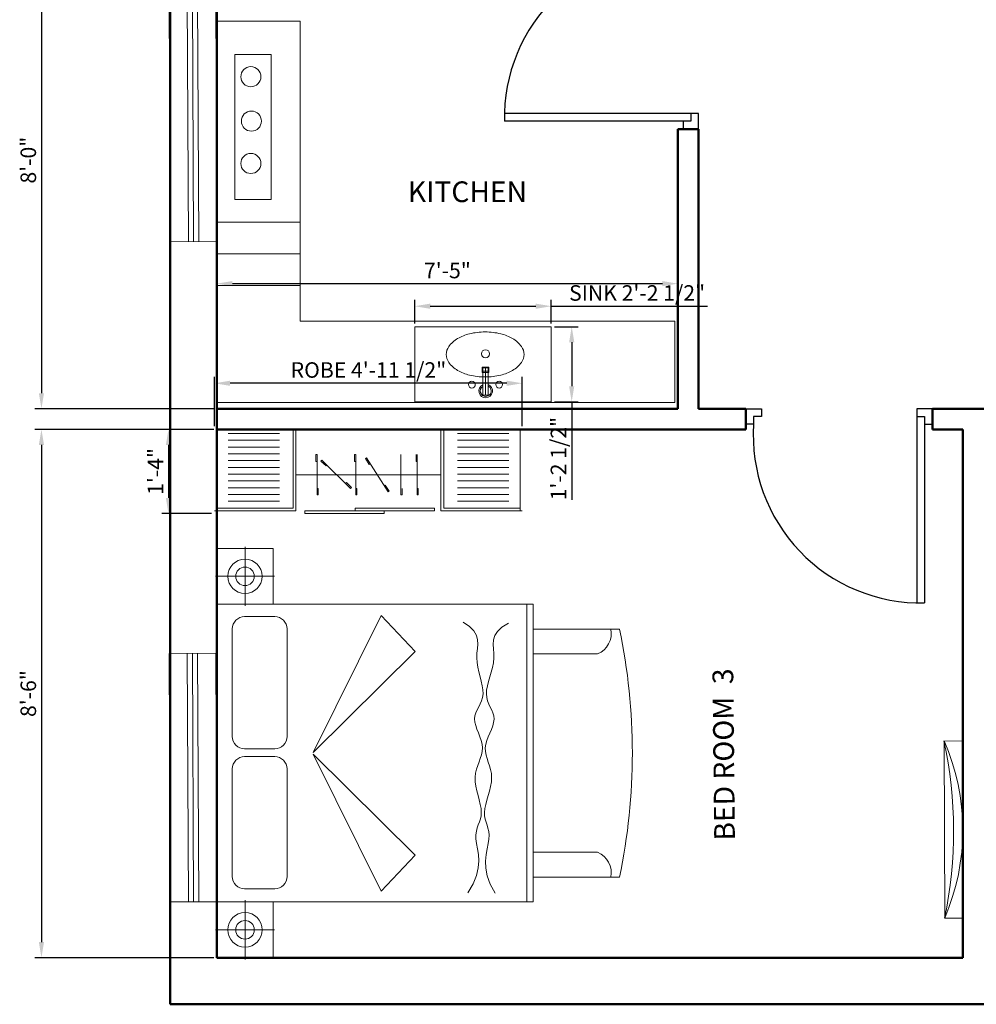
# Model space of a CAD drawing. Units: inches. Extents: x 108 to 1546, y -229 to 513.
# Tile 8 of 11: x 1167 to 1352, y -4 to 187. Entities that reach past the tile are written whole.
import ezdxf

# ---------------------------------------------------------------- set-up
doc = ezdxf.new("R2010")
doc.units = ezdxf.units.IN
for name, color, linetype, lineweight in [('A-ANNO-DIMS', 2, 'Continuous', 18), ('A-AREA-IDEN', 4, 'Continuous', 18), ('A-EQPM', 8, 'Continuous', 18), ('A-FLOR-CBNT', 8, 'Continuous', 18), ('A-FLOR-FIXT', 9, 'Continuous', 18), ('A-FURN', 8, 'Continuous', 13), ('door', 1, 'Continuous', 25), ('tv', 2, 'Continuous', 13), ('wall', 7, 'Continuous', 50), ('WINDOW', 212, 'Continuous', 18)]:
    doc.layers.add(name, color=color, linetype=linetype, lineweight=lineweight)
doc.styles.get("Standard").update_dxf_attribs({"font": 'arial.ttf'})
doc.dimstyles.new('ISO-25', dxfattribs={"dimtxt": 3, "dimasz": 3, "dimexe": 1.25, "dimexo": 0.625, "dimtad": 1, "dimdec": 1, "dimlunit": 3, "dimtxsty": 'Standard', "dimcen": 2.5, "dimadec": 0, "dimazin": 0, "dimtfac": 1, "dimtdec": 1, "dimtmove": 0, "dimatfit": 3, "dimfxl": 1, "dimarcsym": 0})

# ---------------------------------------------------------------- blocks, each defined once
blk = doc.blocks.new('A$C4F543DC7')
for p, q in [((0.0134, 3.35, -0.1688), (3.3134, 3.35, -0.1688)), ((0.4634, 3.35, -0.1688), (0.0134, 3.35, -0.1688)), ((0.0134, 2.896, -0.1688), (0.0134, 3.35, -0.1688)), ((0.0134, 3.35, -0.1688), (0.0134, 2.896, -0.1688)), ((0.2381, 3.1233, -0.4388), (0.2381, 3.3614, -0.4388)), ((0.4634, 3.35, -0.1688), (0.4634, 0.8, -0.1688)), ((2.8634, 3.35, -0.1688), (0.4634, 3.35, -0.1688)), ((0.4634, 2.896, -0.1688), (0.4634, 3.35, -0.1688)), ((2.8634, 0.8, -0.1688), (2.8634, 3.35, -0.1688)), ((2.8634, 3.35, -0.1688), (3.3134, 3.35, -0.1688)), ((2.8634, 2.896, -0.1688), (2.8634, 3.35, -0.1688)), ((3.0888, 3.1233, -0.4388), (3.0888, 3.3614, -0.4388)), ((3.3134, 3.35, -0.1688), (3.3134, 2.896, -0.1688)), ((3.3134, 3.35, -0.1688), (3.3134, 2.896, -0.1688)), ((1.5354, 3.226, -0.1688), (0.6684, 3.226, -0.1688)), ((2.6644, 3.226, -0.1688), (1.7974, 3.226, -0.1688)), ((0.2381, 3.1233, -0.4388), (0, 3.1233, -0.4388)), ((0.2381, 3.1233, -0.4388), (0.4762, 3.1233, -0.4388)), ((0.2381, 3.1233, -0.4388), (0.2381, 2.8852, -0.4388)), ((0.5684, 3.126, -0.1688), (0.5684, 2.884, -0.1688)), ((1.6354, 2.884, -0.1688), (1.6354, 3.126, -0.1688)), ((1.6974, 3.126, -0.1688), (1.6974, 2.884, -0.1688)), ((2.7644, 2.884, -0.1688), (2.7644, 3.126, -0.1688)), ((3.0888, 3.1233, -0.4388), (2.8507, 3.1233, -0.4388)), ((3.0888, 3.1233, -0.4388), (3.0888, 2.8852, -0.4388)), ((3.0888, 3.1233, -0.4388), (3.3269, 3.1233, -0.4388)), ((0.4634, 2.896, -0.1688), (0.0134, 2.896, -0.1688)), ((0.0134, 2.896, -0.1688), (0.4634, 2.896, -0.1688)), ((0.4634, 0.8, -0.1688), (0.4634, 2.896, -0.1688)), ((2.8634, 2.896, -0.1688), (2.8634, 0.8, -0.1688)), ((3.3134, 2.896, -0.1688), (2.8634, 2.896, -0.1688)), ((3.3134, 2.896, -0.1688), (2.8634, 2.896, -0.1688)), ((0.6684, 2.784, -0.1688), (1.5354, 2.784, -0.1688)), ((1.7974, 2.784, -0.1688), (2.6644, 2.784, -0.1688)), ((1.6534, 2.573, -0.1688), (0.5504, 2.025, -0.1688)), ((0.8414, 1.752, -0.1688), (1.6534, 2.573, -0.1688)), ((2.4814, 1.752, -0.1688), (1.6694, 2.573, -0.1688)), ((1.6694, 2.573, -0.1688), (2.7724, 2.025, -0.1688)), ((0.5504, 2.025, -0.1688), (0.8414, 1.752, -0.1688)), ((2.7724, 2.025, -0.1688), (2.4814, 1.752, -0.1688)), ((2.683, 1.312, -0.1688), (2.7182, 1.3641, -0.1688)), ((0.5369, 1.3267, -0.1688), (0.6088, 1.2835, -0.1688)), ((0.6088, 1.2835, -0.1688), (0.6756, 1.2566, -0.1688)), ((1.913, 1.2698, -0.1688), (1.9397, 1.2722, -0.1688)), ((1.9397, 1.2722, -0.1688), (1.9649, 1.2692, -0.1688)), ((2.6129, 1.257, -0.1688), (2.6479, 1.2774, -0.1688)), ((2.6479, 1.2774, -0.1688), (2.683, 1.312, -0.1688)), ((0.6756, 1.2566, -0.1688), (0.7373, 1.2428, -0.1688)), ((0.7373, 1.2428, -0.1688), (0.794, 1.239, -0.1688)), ((0.794, 1.239, -0.1688), (0.8457, 1.242, -0.1688)), ((0.8457, 1.242, -0.1688), (0.8925, 1.2489, -0.1688)), ((0.8925, 1.2489, -0.1688), (0.9345, 1.2564, -0.1688)), ((0.9345, 1.2564, -0.1688), (0.9718, 1.2615, -0.1688)), ((0.9718, 1.2615, -0.1688), (1.0044, 1.2617, -0.1688)), ((1.0044, 1.2617, -0.1688), (1.0334, 1.2578, -0.1688)), ((1.0334, 1.2578, -0.1688), (1.0597, 1.2509, -0.1688)), ((1.0597, 1.2509, -0.1688), (1.0842, 1.2424, -0.1688)), ((1.0842, 1.2424, -0.1688), (1.1081, 1.2336, -0.1688)), ((1.1081, 1.2336, -0.1688), (1.1322, 1.2257, -0.1688)), ((1.1316, 1.1872, -0.1688), (1.1573, 1.192, -0.1688)), ((1.1322, 1.2257, -0.1688), (1.1577, 1.2201, -0.1688)), ((1.1573, 1.192, -0.1688), (1.1851, 1.1932, -0.1688)), ((1.1577, 1.2201, -0.1688), (1.1855, 1.218, -0.1688)), ((1.1851, 1.1932, -0.1688), (1.2158, 1.1898, -0.1688)), ((1.1855, 1.218, -0.1688), (1.2163, 1.2204, -0.1688)), ((1.2163, 1.2204, -0.1688), (1.2498, 1.2264, -0.1688)), ((1.2498, 1.2264, -0.1688), (1.2852, 1.2347, -0.1688)), ((1.2852, 1.2347, -0.1688), (1.3218, 1.2441, -0.1688)), ((1.3218, 1.2441, -0.1688), (1.3591, 1.2533, -0.1688)), ((1.3591, 1.2533, -0.1688), (1.3963, 1.2612, -0.1688)), ((1.3963, 1.2612, -0.1688), (1.4328, 1.2664, -0.1688)), ((1.4328, 1.2664, -0.1688), (1.4679, 1.2677, -0.1688)), ((1.4679, 1.2677, -0.1688), (1.501, 1.2643, -0.1688)), ((1.501, 1.2643, -0.1688), (1.5324, 1.257, -0.1688)), ((1.5324, 1.257, -0.1688), (1.5624, 1.2473, -0.1688)), ((1.5624, 1.2473, -0.1688), (1.5915, 1.2365, -0.1688)), ((1.5915, 1.2365, -0.1688), (1.6199, 1.2259, -0.1688)), ((1.6199, 1.2259, -0.1688), (1.6481, 1.2169, -0.1688)), ((1.6481, 1.2169, -0.1688), (1.6765, 1.2108, -0.1688)), ((1.6765, 1.2108, -0.1688), (1.7053, 1.209, -0.1688)), ((1.7053, 1.209, -0.1688), (1.7349, 1.2124, -0.1688)), ((1.7349, 1.2124, -0.1688), (1.7651, 1.2199, -0.1688)), ((1.7651, 1.2199, -0.1688), (1.7955, 1.2301, -0.1688)), ((1.7955, 1.2301, -0.1688), (1.8258, 1.2417, -0.1688)), ((1.8258, 1.2417, -0.1688), (1.8557, 1.2531, -0.1688)), ((1.8557, 1.2531, -0.1688), (1.8849, 1.263, -0.1688)), ((1.8849, 1.263, -0.1688), (1.913, 1.2698, -0.1688)), ((1.9649, 1.2692, -0.1688), (1.989, 1.2617, -0.1688)), ((1.989, 1.2617, -0.1688), (2.0124, 1.2512, -0.1688)), ((2.0124, 1.2512, -0.1688), (2.0359, 1.2391, -0.1688)), ((2.0359, 1.2391, -0.1688), (2.0599, 1.2269, -0.1688)), ((2.0599, 1.2269, -0.1688), (2.0849, 1.216, -0.1688)), ((2.0849, 1.216, -0.1688), (2.1117, 1.2077, -0.1688)), ((2.1117, 1.2077, -0.1688), (2.1407, 1.2037, -0.1688)), ((2.1407, 1.2037, -0.1688), (2.1723, 1.2047, -0.1688)), ((2.1723, 1.2047, -0.1688), (2.2062, 1.21, -0.1688)), ((2.2062, 1.21, -0.1688), (2.242, 1.2182, -0.1688)), ((2.242, 1.2182, -0.1688), (2.2791, 1.2279, -0.1688)), ((2.2791, 1.2279, -0.1688), (2.3173, 1.2378, -0.1688)), ((2.3173, 1.2378, -0.1688), (2.3558, 1.2465, -0.1688)), ((2.3558, 1.2465, -0.1688), (2.3944, 1.2527, -0.1688)), ((2.3944, 1.2527, -0.1688), (2.4325, 1.255, -0.1688)), ((2.4325, 1.255, -0.1688), (2.4698, 1.2529, -0.1688)), ((2.4698, 1.2529, -0.1688), (2.5064, 1.2488, -0.1688)), ((2.5064, 1.2488, -0.1688), (2.5423, 1.2459, -0.1688)), ((2.5423, 1.2459, -0.1688), (2.5777, 1.2476, -0.1688)), ((2.5777, 1.2476, -0.1688), (2.6129, 1.257, -0.1688)), ((0.5334, 1.105, -0.1688), (0.6067, 1.1458, -0.1688)), ((0.6067, 1.1458, -0.1688), (0.6743, 1.1706, -0.1688)), ((0.6743, 1.1706, -0.1688), (0.7364, 1.1825, -0.1688)), ((0.7364, 1.1825, -0.1688), (0.7931, 1.1846, -0.1688)), ((0.7931, 1.1846, -0.1688), (0.8447, 1.1799, -0.1688)), ((0.8447, 1.1799, -0.1688), (0.8913, 1.1716, -0.1688)), ((0.8913, 1.1716, -0.1688), (0.9331, 1.1628, -0.1688)), ((0.9331, 1.1628, -0.1688), (0.9701, 1.1565, -0.1688)), ((0.9701, 1.1565, -0.1688), (1.0027, 1.1552, -0.1688)), ((1.0027, 1.1552, -0.1688), (1.0318, 1.1582, -0.1688)), ((1.0318, 1.1582, -0.1688), (1.0583, 1.1642, -0.1688)), ((1.0583, 1.1642, -0.1688), (1.0831, 1.172, -0.1688)), ((1.0831, 1.172, -0.1688), (1.1072, 1.18, -0.1688)), ((1.1072, 1.18, -0.1688), (1.1316, 1.1872, -0.1688)), ((1.2158, 1.1898, -0.1688), (1.2491, 1.1828, -0.1688)), ((1.2491, 1.1828, -0.1688), (1.2842, 1.1734, -0.1688)), ((1.2842, 1.1734, -0.1688), (1.3206, 1.1629, -0.1688)), ((1.3206, 1.1629, -0.1688), (1.3575, 1.1524, -0.1688)), ((1.3575, 1.1524, -0.1688), (1.3945, 1.1434, -0.1688)), ((1.3945, 1.1434, -0.1688), (1.4308, 1.1371, -0.1688)), ((1.4308, 1.1371, -0.1688), (1.4658, 1.1347, -0.1688)), ((1.4658, 1.1347, -0.1688), (1.499, 1.137, -0.1688)), ((1.499, 1.137, -0.1688), (1.5306, 1.1433, -0.1688)), ((1.5306, 1.1433, -0.1688), (1.5609, 1.152, -0.1688)), ((1.5609, 1.152, -0.1688), (1.5903, 1.1619, -0.1688)), ((1.5903, 1.1619, -0.1688), (1.6191, 1.1716, -0.1688)), ((1.6191, 1.1716, -0.1688), (1.6475, 1.1797, -0.1688)), ((1.6475, 1.1797, -0.1688), (1.676, 1.1849, -0.1688)), ((1.676, 1.1849, -0.1688), (1.7049, 1.1858, -0.1688)), ((1.7049, 1.1858, -0.1688), (1.7344, 1.1816, -0.1688)), ((1.7344, 1.1816, -0.1688), (1.7643, 1.1731, -0.1688)), ((1.7643, 1.1731, -0.1688), (1.7944, 1.1619, -0.1688)), ((1.7944, 1.1619, -0.1688), (1.8244, 1.1494, -0.1688)), ((1.8244, 1.1494, -0.1688), (1.8539, 1.137, -0.1688)), ((1.8539, 1.137, -0.1688), (1.8827, 1.1263, -0.1688)), ((1.8827, 1.1263, -0.1688), (1.9106, 1.1186, -0.1688)), ((1.9106, 1.1186, -0.1688), (1.9373, 1.1153, -0.1688)), ((1.9373, 1.1153, -0.1688), (1.9625, 1.1176, -0.1688)), ((1.9625, 1.1176, -0.1688), (1.9868, 1.1243, -0.1688)), ((1.9868, 1.1243, -0.1688), (2.0106, 1.134, -0.1688)), ((2.0106, 1.134, -0.1688), (2.0344, 1.1454, -0.1688)), ((2.0344, 1.1454, -0.1688), (2.0588, 1.1568, -0.1688)), ((2.0588, 1.1568, -0.1688), (2.0842, 1.167, -0.1688)), ((2.0842, 1.167, -0.1688), (2.1112, 1.1743, -0.1688)), ((2.1112, 1.1743, -0.1688), (2.1403, 1.1775, -0.1688)), ((2.1403, 1.1775, -0.1688), (2.1718, 1.1755, -0.1688)), ((2.1718, 1.1755, -0.1688), (2.2056, 1.1691, -0.1688)), ((2.2056, 1.1691, -0.1688), (2.2411, 1.1598, -0.1688)), ((2.2411, 1.1598, -0.1688), (2.2779, 1.1489, -0.1688)), ((2.2779, 1.1489, -0.1688), (2.3157, 1.1379, -0.1688)), ((2.3157, 1.1379, -0.1688), (2.354, 1.1279, -0.1688)), ((2.354, 1.1279, -0.1688), (2.3923, 1.1205, -0.1688)), ((2.3923, 1.1205, -0.1688), (2.4304, 1.117, -0.1688)), ((2.4304, 1.117, -0.1688), (2.4677, 1.118, -0.1688)), ((2.4677, 1.118, -0.1688), (2.5043, 1.1209, -0.1688)), ((2.5043, 1.1209, -0.1688), (2.5403, 1.1226, -0.1688)), ((2.5403, 1.1226, -0.1688), (2.5757, 1.1199, -0.1688)), ((2.5757, 1.1199, -0.1688), (2.6106, 1.1094, -0.1688)), ((2.6106, 1.1094, -0.1688), (2.645, 1.0879, -0.1688)), ((2.645, 1.0879, -0.1688), (2.6789, 1.0522, -0.1688)), ((2.6789, 1.0522, -0.1688), (2.7124, 0.999, -0.1688)), ((0.4634, 0.85, -0.1688), (2.8634, 0.85, -0.1688)), ((0.4634, 0.8, -0.1688), (2.8634, 0.8, -0.1688)), ((0.6634, 0.8, -0.1688), (0.4634, 0.8, -0.1688)), ((0.6634, 0.8, -0.1688), (2.6634, 0.8, -0.1688)), ((0.6634, 0.104, -0.1688), (0.6634, 0.8, -0.1688)), ((0.6634, 0.104, -0.1688), (0.6634, 0.8, -0.1688)), ((0.8634, 0.281, -0.1688), (0.8634, 0.8, -0.1688)), ((2.4634, 0.8, -0.1688), (2.4634, 0.281, -0.1688)), ((2.8634, 0.8, -0.1688), (2.6634, 0.8, -0.1688)), ((2.6634, 0.8, -0.1688), (2.6634, 0.104, -0.1688)), ((2.6634, 0.8, -0.1688), (2.6634, 0.104, -0.1688))]:
    blk.add_line(p, q)
for centre, radius in [((0.2381, 3.1233, -0.4388), 0.139), ((3.0888, 3.1233, -0.4388), 0.139), ((0.2381, 3.1233, -0.4388), 0.075), ((3.0888, 3.1233, -0.4388), 0.075)]:
    blk.add_circle(centre, radius)
for centre, radius, start, end in [((0.6684, 3.126, -0.1688), 0.1, 90, 180), ((1.5354, 3.126, -0.1688), 0.1, 0, 90), ((1.7974, 3.126, -0.1688), 0.1, 90, 180), ((2.6644, 3.126, -0.1688), 0.1, 0, 90), ((0.6684, 2.884, -0.1688), 0.1, 180, 270), ((1.5354, 2.884, -0.1688), 0.1, 270, 0), ((1.7974, 2.884, -0.1688), 0.1, 180, 270), ((2.6644, 2.884, -0.1688), 0.1, 270, 0), ((0.6994, 0.3472, -0.1688), 0.1769, 258.2616, 338.03196), ((2.6275, 0.3472, -0.1688), 0.1769, 201.96804, 281.7384), ((1.6634, 4.8597, -0.1688), 4.8597, 258.12517, 281.87483), ((1.6634, 4.8597, -0.1688), 4.8597, 258.12517, 281.87483)]:
    blk.add_arc(centre, radius, start, end)
blk = doc.blocks.new('A$C34930FF8')
at = {"ltscale": 0.05}
for p, q in [((0, 2252.4), (0, 16.8)), ((600, 2252.4), (0, 2252.4)), ((185.4, 1513), (185.4, 1521.5)), ((227.1, 1479.2), (233.2, 1485.2)), ((237.7, 1513), (237.7, 1521.5)), ((436.7, 1513), (436.7, 1504.4)), ((482.5, 1513), (482.5, 1504.4)), ((263.6, 1441.7), (269.7, 1447.7)), ((185.4, 1229.1), (185.4, 1237.7)), ((237.7, 1229.1), (237.7, 1237.7)), ((398.2, 1303.6), (392.1, 1297.6)), ((434.8, 1266.1), (428.7, 1260.1)), ((436.7, 1228.2), (436.7, 1219.7)), ((482.5, 1228.2), (482.5, 1219.7)), ((209.5, 1150.1), (214.1, 1157.3)), ((253.5, 1121.8), (258.1, 1129)), ((415.3, 1017.6), (410.6, 1010.5)), ((459.3, 989.3), (454.7, 982.1)), ((482.5, 894.9), (482.5, 886.3)), ((237.7, 775.3), (237.7, 783.9)), ((436.7, 775.3), (436.7, 766.8)), ((482.5, 775.3), (482.5, 766.8)), ((600, 16.8), (0, 16.8))]:
    blk.add_line(p, q, dxfattribs=at)
for p, q in [((580, 1690.9), (580, 2252.4)), ((600, 1669.3), (600, 2269.3)), ((30, 1790.9), (30, 2169.3)), ((80, 1790.9), (80, 2169.3)), ((130, 1790.9), (130, 2169.3)), ((180, 1790.9), (180, 2169.3)), ((230, 1790.9), (230, 2169.3)), ((280, 1790.9), (280, 2169.3)), ((330, 1790.9), (330, 2169.3)), ((380, 1790.9), (380, 2169.3)), ((430, 1790.9), (430, 2169.3)), ((480, 1790.9), (480, 2169.3)), ((530, 1790.9), (530, 2169.3)), ((580, 1690.9), (0, 1690.9)), ((600, 1669.3), (0, 1669.3)), ((335.4, 1666.1), (335.4, 603.1)), ((600, 1603.3), (620, 1603.3)), ((600, 1018.7), (600, 1603.3)), ((620, 1603.3), (620, 1018.7)), ((237.7, 1521.5), (185.4, 1521.5)), ((482.5, 1513), (185.4, 1513)), ((434.8, 1266.1), (227.4, 1478.9)), ((269.7, 1447.7), (233.2, 1485.2)), ((436.7, 1504.4), (482.5, 1504.4)), ((237.7, 1237.7), (185.4, 1237.7)), ((428.7, 1260.1), (392.1, 1297.6)), ((482.5, 1228.2), (185.4, 1228.2)), ((436.7, 1219.7), (482.5, 1219.7)), ((600, 1233.4), (580, 1233.4)), ((580, 1233.4), (580, 648.7)), ((600, 648.7), (600, 1233.4)), ((459.3, 989.3), (209.5, 1150.1)), ((258.1, 1129), (214.1, 1157.3)), ((620, 1018.7), (600, 1018.7)), ((454.7, 982.1), (410.6, 1010.5)), ((482.5, 894.9), (185.4, 894.9)), ((436.7, 886.3), (482.5, 886.3)), ((237.7, 783.9), (185.4, 783.9)), ((482.5, 775.3), (185.4, 775.3)), ((436.7, 766.8), (482.5, 766.8)), ((600, 600), (0, 600)), ((580, 648.7), (600, 648.7)), ((600, 600), (600, 0)), ((580, 578.3), (0, 578.3)), ((580, 578.3), (580, 16.8)), ((30, 478.3), (30, 100)), ((80, 478.3), (80, 100)), ((130, 478.3), (130, 100)), ((180, 478.3), (180, 100)), ((230, 478.3), (230, 100)), ((280, 478.3), (280, 100)), ((330, 478.3), (330, 100)), ((380, 478.3), (380, 100)), ((430, 478.3), (430, 100)), ((480, 478.3), (480, 100)), ((530, 478.3), (530, 100))]:
    blk.add_line(p, q)
blk = doc.blocks.new('A$C50A015BB')
for p, q in [((0, 0.55), (1, 0.55)), ((0, 0.55), (0, 0)), ((1, 0.55), (1, 0)), ((0.4985, 0.5), (0.5385, 0.5)), ((0.4985, 0.5), (0.4985, 0.3)), ((0.5185, 0.5), (0.5185, 0.3)), ((0.5385, 0.5), (0.5385, 0.3)), ((0.4935, 0.335), (0.4935, 0.295)), ((0.4935, 0.335), (0.5435, 0.335)), ((0.4935, 0.295), (0.5435, 0.295)), ((0.4985, 0.325), (0.5385, 0.325)), ((0.4985, 0.3), (0.5385, 0.3)), ((0.5435, 0.335), (0.5435, 0.295)), ((0, 0), (1, 0)), ((0, 0), (1, 0))]:
    blk.add_line(p, q)
for centre, radius in [((0.4185, 0.424), 0.025), ((0.6185, 0.424), 0.025), ((0.5185, 0.1981), 0.0298)]:
    blk.add_circle(centre, radius)
for centre, radius, start, end in [((0.5201, 0.4703), 0.0497, 291.74253, 244.23308), ((0.5201, 0.4703), 0.0397, 297.63203, 237.02558), ((0.5157, -0.1225), 0.4906, 90, 103.48533), ((0.5157, -0.1225), 0.4906, 76.51467, 90), ((0.4185, 0.1397), 0.2081, 120.06859, 144.41781), ((0.4772, 0.0383), 0.3252, 103.48533, 120.06859), ((0.5543, 0.0383), 0.3252, 59.93141, 76.51467), ((0.613, 0.1397), 0.2081, 35.58219, 59.93141), ((0.3299, 0.2031), 0.0991, 144.41781, 180), ((0.7016, 0.2031), 0.0991, 0, 35.58219), ((0.3299, 0.2031), 0.0991, 180, 215.58219), ((0.4185, 0.2665), 0.2081, 215.58219, 239.93141), ((0.613, 0.2665), 0.2081, 300.06859, 324.41781), ((0.7016, 0.2031), 0.0991, 324.41781, 0), ((0.4772, 0.3679), 0.3252, 239.93141, 256.51467), ((0.5543, 0.3679), 0.3252, 283.48533, 300.06859), ((0.5157, 0.5288), 0.4906, 256.51467, 270), ((0.5157, 0.5288), 0.4906, 270, 283.48533)]:
    blk.add_arc(centre, radius, start, end)
blk = doc.blocks.new('WINDOW-48X9')
for p, q in [((0, 9), (0, 0)), ((0, 9), (48, 9)), ((48, 9), (48, 0)), ((0, 5.5), (48, 5.5)), ((0, 4.5), (48, 4.5)), ((0, 3.5), (48, 3.5)), ((0, 0), (48, 0))]:
    blk.add_line(p, q)
blk = doc.blocks.new('DOOR-SWING-36')
for p, q in [((1.5, 1.5), (1.5, 37.5)), ((3, 1.5), (3, 37.5)), ((0, 3), (0, 0)), ((1.5, 3), (0, 3)), ((1.5, 1.5), (1.5, 3)), ((34.5, 1.5), (34.5, 3)), ((34.5, 3), (36, 3)), ((36, 3), (36, 0)), ((3, 1.5), (1.5, 1.5)), ((3, 0), (3, 1.5)), ((33, 0), (33, 1.5)), ((33, 1.5), (34.5, 1.5)), ((0, 0), (3, 0)), ((36, 0), (33, 0))]:
    blk.add_line(p, q)
blk.add_arc((2.25, 5.18), 32.32, 356.1244, 91.3295)
blk = doc.blocks.new('TV-WALL-MOUNT')
blk.add_lwpolyline([(0, 0), (34.19, 0), (34.19, 3.56), (0, 3.56)], close=True)
for centre, radius, start, end in [((17.1, 42.8), 42.8, 246.4582, 293.5418), ((17.1, 84.72), 82.93, 258.1036, 281.8964)]:
    blk.add_arc(centre, radius, start, end)
blk = doc.blocks.new('*D46')
at = {"layer": 'A-ANNO-DIMS', "color": 0, "lineweight": -2, "transparency": 16777216}
for p, q in [((1204.5, 108.09), (1204.5, 117.63)), ((1260.9, 116.38), (1207.5, 116.38)), ((1263.9, 108.09), (1263.9, 117.63))]:
    blk.add_line(p, q, dxfattribs=at)
at = {"layer": 'A-ANNO-DIMS', "color": 0, "transparency": 16777216}
for points in [[(1207.5, 116.88), (1207.5, 115.88), (1204.5, 116.38)], [(1260.9, 116.88), (1260.9, 115.88), (1263.9, 116.38)]]:
    blk.add_solid(points, dxfattribs=at)
at = {"layer": 'Defpoints', "color": 0, "transparency": 16777216}
for p in [(1204.5, 116.38), (1204.5, 107.47), (1263.9, 107.47)]:
    blk.add_point(p, dxfattribs=at)
at = {"layer": 'A-ANNO-DIMS', "color": 0, "transparency": 16777216, "insert": (1234.2, 118.56), "char_height": 3, "attachment_point": 5}
blk.add_mtext('ROBE 4\'-11 1/2"', dxfattribs=at)
blk = doc.blocks.new('*D47')
at = {"layer": 'A-ANNO-DIMS', "color": 0, "lineweight": -2, "transparency": 16777216}
for p, q in [((1203.87, 107.47), (1194.34, 107.47)), ((1195.59, 104.47), (1195.59, 94.24)), ((1203.87, 91.24), (1194.34, 91.24))]:
    blk.add_line(p, q, dxfattribs=at)
at = {"layer": 'A-ANNO-DIMS', "color": 0, "transparency": 16777216}
for points in [[(1195.09, 104.47), (1196.09, 104.47), (1195.59, 107.47)], [(1195.09, 94.24), (1196.09, 94.24), (1195.59, 91.24)]]:
    blk.add_solid(points, dxfattribs=at)
at = {"layer": 'Defpoints', "color": 0, "transparency": 16777216}
for p in [(1204.5, 107.47), (1195.59, 91.24), (1204.5, 91.24)]:
    blk.add_point(p, dxfattribs=at)
at = {"layer": 'A-ANNO-DIMS', "color": 0, "transparency": 16777216, "insert": (1193.46, 99.36), "char_height": 3, "attachment_point": 5, "rotation": 90}
blk.add_mtext('1\'-4"', dxfattribs=at)
blk = doc.blocks.new('*D58')
at = {"layer": 'A-ANNO-DIMS', "color": 0, "lineweight": -2, "transparency": 16777216}
for p, q in [((1243.13, 127.93), (1243.13, 132.51)), ((1246.13, 131.26), (1266.49, 131.26)), ((1269.49, 127.93), (1269.49, 132.51)), ((1269.49, 131.26), (1299.64, 131.26))]:
    blk.add_line(p, q, dxfattribs=at)
at = {"layer": 'A-ANNO-DIMS', "color": 0, "transparency": 16777216}
for points in [[(1246.13, 131.76), (1246.13, 130.76), (1243.13, 131.26)], [(1266.49, 131.76), (1266.49, 130.76), (1269.49, 131.26)]]:
    blk.add_solid(points, dxfattribs=at)
at = {"layer": 'Defpoints', "color": 0, "transparency": 16777216}
for p in [(1269.49, 131.26), (1243.13, 127.3), (1269.49, 127.3)]:
    blk.add_point(p, dxfattribs=at)
at = {"layer": 'A-ANNO-DIMS', "color": 0, "transparency": 16777216, "insert": (1286.06, 133.43), "char_height": 3, "attachment_point": 5}
blk.add_mtext('SINK 2\'-2 1/2"', dxfattribs=at)
blk = doc.blocks.new('*D59')
at = {"layer": 'A-ANNO-DIMS', "color": 0, "lineweight": -2, "transparency": 16777216}
for p, q in [((1270.11, 127.3), (1274.69, 127.3)), ((1273.44, 124.3), (1273.44, 115.8)), ((1270.11, 112.8), (1274.69, 112.8)), ((1273.44, 112.8), (1273.44, 93.87))]:
    blk.add_line(p, q, dxfattribs=at)
at = {"layer": 'A-ANNO-DIMS', "color": 0, "transparency": 16777216}
for points in [[(1272.94, 124.3), (1273.94, 124.3), (1273.44, 127.3)], [(1272.94, 115.8), (1273.94, 115.8), (1273.44, 112.8)]]:
    blk.add_solid(points, dxfattribs=at)
at = {"layer": 'Defpoints', "color": 0, "transparency": 16777216}
for p in [(1269.49, 127.3), (1269.49, 112.8), (1273.44, 112.8)]:
    blk.add_point(p, dxfattribs=at)
at = {"layer": 'A-ANNO-DIMS', "color": 0, "transparency": 16777216, "insert": (1271.27, 101.84), "char_height": 3, "attachment_point": 5, "rotation": 90}
blk.add_mtext('1\'-2 1/2"', dxfattribs=at)
blk = doc.blocks.new('*D104')
at = {"layer": 'A-ANNO-DIMS', "color": 0, "lineweight": -2, "transparency": 16777216}
for p, q in [((1204.94, 112.09), (1204.94, 136.87)), ((1207.94, 135.62), (1290.94, 135.62)), ((1293.94, 112.09), (1293.94, 136.87))]:
    blk.add_line(p, q, dxfattribs=at)
at = {"layer": 'A-ANNO-DIMS', "color": 0, "transparency": 16777216}
for points in [[(1207.94, 136.12), (1207.94, 135.12), (1204.94, 135.62)], [(1290.94, 136.12), (1290.94, 135.12), (1293.94, 135.62)]]:
    blk.add_solid(points, dxfattribs=at)
at = {"layer": 'Defpoints', "color": 0, "transparency": 16777216}
for p in [(1293.94, 135.62), (1204.94, 111.47), (1293.94, 111.47)]:
    blk.add_point(p, dxfattribs=at)
at = {"layer": 'A-ANNO-DIMS', "color": 0, "transparency": 16777216, "insert": (1249.44, 137.77), "char_height": 3, "attachment_point": 5}
blk.add_mtext('7\'-5"', dxfattribs=at)
blk = doc.blocks.new('*D107')
at = {"layer": 'A-ANNO-DIMS', "color": 0, "lineweight": -2, "transparency": 16777216}
for p, q in [((1204.32, 207.47), (1169.82, 207.47)), ((1171.07, 204.47), (1171.07, 114.47)), ((1204.32, 111.47), (1169.82, 111.47))]:
    blk.add_line(p, q, dxfattribs=at)
at = {"layer": 'A-ANNO-DIMS', "color": 0, "transparency": 16777216}
for points in [[(1170.57, 204.47), (1171.57, 204.47), (1171.07, 207.47)], [(1170.57, 114.47), (1171.57, 114.47), (1171.07, 111.47)]]:
    blk.add_solid(points, dxfattribs=at)
at = {"layer": 'Defpoints', "color": 0, "transparency": 16777216}
for p in [(1204.94, 207.47), (1171.07, 111.47), (1204.94, 111.47)]:
    blk.add_point(p, dxfattribs=at)
at = {"layer": 'A-ANNO-DIMS', "color": 0, "transparency": 16777216, "insert": (1168.92, 159.47), "char_height": 3, "attachment_point": 5, "rotation": 90}
blk.add_mtext('8\'-0"', dxfattribs=at)
blk = doc.blocks.new('*D108')
at = {"layer": 'A-ANNO-DIMS', "color": 0, "lineweight": -2, "transparency": 16777216}
for p, q in [((1204.32, 107.47), (1169.82, 107.47)), ((1171.07, 104.47), (1171.07, 8.47)), ((1204.32, 5.47), (1169.82, 5.47))]:
    blk.add_line(p, q, dxfattribs=at)
at = {"layer": 'A-ANNO-DIMS', "color": 0, "transparency": 16777216}
for points in [[(1170.57, 104.47), (1171.57, 104.47), (1171.07, 107.47)], [(1170.57, 8.47), (1171.57, 8.47), (1171.07, 5.47)]]:
    blk.add_solid(points, dxfattribs=at)
at = {"layer": 'Defpoints', "color": 0, "transparency": 16777216}
for p in [(1204.94, 107.47), (1171.07, 5.47), (1204.94, 5.47)]:
    blk.add_point(p, dxfattribs=at)
at = {"layer": 'A-ANNO-DIMS', "color": 0, "transparency": 16777216, "insert": (1168.92, 56.47), "char_height": 3, "attachment_point": 5, "rotation": 90}
blk.add_mtext('8\'-6"', dxfattribs=at)

msp = doc.modelspace()

# ---------------------------------------------------------------- linework, layer by layer
at = {"layer": 'A-EQPM'}
msp.add_lwpolyline([(1208.38, 179.89), (1215.4, 179.89), (1215.4, 151.84), (1208.38, 151.84)], close=True, dxfattribs=at)
for centre in [(1211.5, 175.58), (1211.6, 167.01), (1211.5, 158.83)]:
    msp.add_circle(centre, 1.94, dxfattribs=at)
at = {"layer": 'A-FLOR-CBNT'}
for p, q in [((1204.94, 186.33), (1220.99, 186.33)), ((1204.94, 112.68), (1204.94, 186.33)), ((1220.99, 186.33), (1220.99, 128.37)), ((1204.94, 141.37), (1220.99, 141.37)), ((1293.33, 128.37), (1220.99, 128.37)), ((1293.33, 112.68), (1293.33, 128.37)), ((1204.94, 112.68), (1293.33, 112.68))]:
    msp.add_line(p, q, dxfattribs=at)
msp.add_lwpolyline([(1204.94, 147.49), (1220.99, 147.49), (1220.99, 135.25), (1204.94, 135.25)], close=True, dxfattribs=at)
at = {"layer": 'wall'}
for p, q in [((1195.94, 452.47), (1195.94, -3.53)), ((1204.94, 443.47), (1204.94, 5.47)), ((1293.94, 165.47), (1297.94, 165.47)), ((1293.94, 165.47), (1293.94, 111.47)), ((1297.94, 165.47), (1297.94, 111.47)), ((1293.94, 111.47), (1204.94, 111.47)), ((1307.06, 111.47), (1297.94, 111.47)), ((1307.06, 111.47), (1307.06, 107.47)), ((1343.06, 111.47), (1343.06, 107.47)), ((1358.94, 111.47), (1343.06, 111.47)), ((1307.06, 107.47), (1204.94, 107.47)), ((1348.94, 107.47), (1343.06, 107.47)), ((1348.94, 107.47), (1348.94, 5.47)), ((1204.94, 5.47), (1348.94, 5.47)), ((1195.94, -3.53), (1519.94, -3.53))]:
    msp.add_line(p, q, dxfattribs=at)

# ---------------------------------------------------------------- block references
at = {"layer": 'A-FLOR-FIXT', "xscale": -26.36213054902417, "yscale": 26.36213054902417, "zscale": 26.36213054902417, "rotation": 180}
msp.add_blockref('A$C50A015BB', (1243.13, 127.3), dxfattribs=at)
at = {"layer": 'A-FURN', "rotation": 90}
for name, p, xscale, yscale, zscale in [('A$C34930FF8', (1263.9, 107.47), -0.0261767283193444, 0.0261767283193444, 0.0261767283193444), ('A$C4F543DC7', (1285.15, 5.15, 4.04), 23.94379789781286, 23.94379789781286, 23.94379789781286)]:
    msp.add_blockref(name, p, dxfattribs=dict(at, xscale=xscale, yscale=yscale, zscale=zscale))
at = {"layer": 'door'}
for p, rotation in [((1297.94, 165.47), 90.00000000000017), ((1343.06, 111.47), 180)]:
    msp.add_blockref('DOOR-SWING-36', p, dxfattribs=dict(at, rotation=rotation))
at = {"layer": 'tv', "rotation": 90.20656548976669}
msp.add_blockref('TV-WALL-MOUNT', (1349, 13.13), dxfattribs=at)
at = {"layer": 'WINDOW'}
for p, rotation in [((1204.94, 143.74), 90.27995600980967), ((1204.94, 16.28), 90.27995600980968)]:
    msp.add_blockref('WINDOW-48X9', p, dxfattribs=dict(at, rotation=rotation))

# ---------------------------------------------------------------- texts
at = {"layer": 'A-AREA-IDEN', "insert": (1241.81, 155.36), "char_height": 4, "attachment_point": 1}
msp.add_mtext_dynamic_manual_height_columns('KITCHEN', width=57.4311, gutter_width=12.5, heights=[12.84], dxfattribs=at)
at = {"layer": 'A-AREA-IDEN', "insert": (1300.95, 28.06), "char_height": 4, "attachment_point": 1, "rotation": 90.5856}
msp.add_mtext_dynamic_manual_height_columns('BED ROOM  3', width=57.4311, gutter_width=12.5, heights=[12.84], dxfattribs=at)

# ---------------------------------------------------------------- dimensions: what is measured, and where the dimension line sits
at = {"layer": 'A-ANNO-DIMS'}
for base, p1, p2, angle, picture, middle in [((1171.07, 111.47), (1204.94, 207.47), (1204.94, 111.47), 90, '*D107', (1168.92, 159.47)), ((1273.44, 112.8), (1269.49, 127.3), (1269.49, 112.8), 270, '*D59', (1271.27, 101.84)), ((1171.07, 5.47), (1204.94, 107.47), (1204.94, 5.47), 90, '*D108', (1168.92, 56.47)), ((1195.59, 91.24), (1204.5, 107.47), (1204.5, 91.24), 270, '*D47', (1193.46, 99.36))]:
    dim = msp.add_linear_dim(base=base, p1=p1, p2=p2, angle=angle, dimstyle='ISO-25', override={"dimdec": 1, "dimlfac": 1, "dimrnd": 0, "dimzin": 1, "dimdsep": 46, "dimlunit": 4, "dimfrac": 2}, dxfattribs=at)
    dim.commit()
    dim.dimension.update_dxf_attribs({"geometry": picture, "text_midpoint": middle})
dim = msp.add_linear_dim(base=(1293.94, 135.62), p1=(1204.94, 111.47), p2=(1293.94, 111.47), dimstyle='ISO-25', override={"dimdec": 1, "dimlfac": 1, "dimrnd": 0, "dimzin": 1, "dimdsep": 46, "dimlunit": 4, "dimfrac": 2}, dxfattribs=at)
dim.commit()
dim.dimension.update_dxf_attribs({"geometry": '*D104', "text_midpoint": (1249.44, 137.77)})
dim = msp.add_linear_dim(base=(1269.49, 131.26), p1=(1243.13, 127.3), p2=(1269.49, 127.3), text='SINK <>', dimstyle='ISO-25', override={"dimdec": 1, "dimlfac": 1, "dimrnd": 0, "dimzin": 1, "dimdsep": 46, "dimlunit": 4, "dimfrac": 2}, dxfattribs=at)
dim.commit()
dim.dimension.update_dxf_attribs({"geometry": '*D58', "text_midpoint": (1286.06, 133.43)})
dim = msp.add_linear_dim(base=(1204.5, 116.38), p1=(1263.9, 107.47), p2=(1204.5, 107.47), angle=180, text='ROBE <>', dimstyle='ISO-25', override={"dimdec": 1, "dimlfac": 1, "dimrnd": 0, "dimzin": 1, "dimdsep": 46, "dimlunit": 4, "dimfrac": 2}, dxfattribs=at)
dim.commit()
dim.dimension.update_dxf_attribs({"geometry": '*D46', "text_midpoint": (1234.2, 118.56)})

doc.saveas('drawing.dxf')
